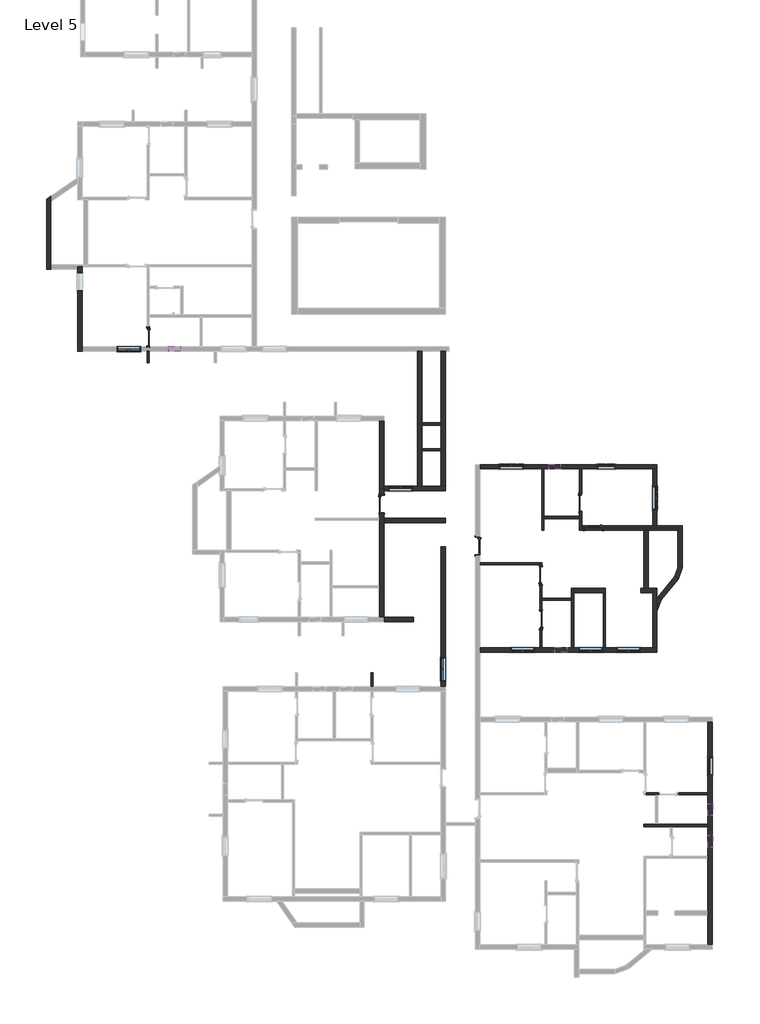
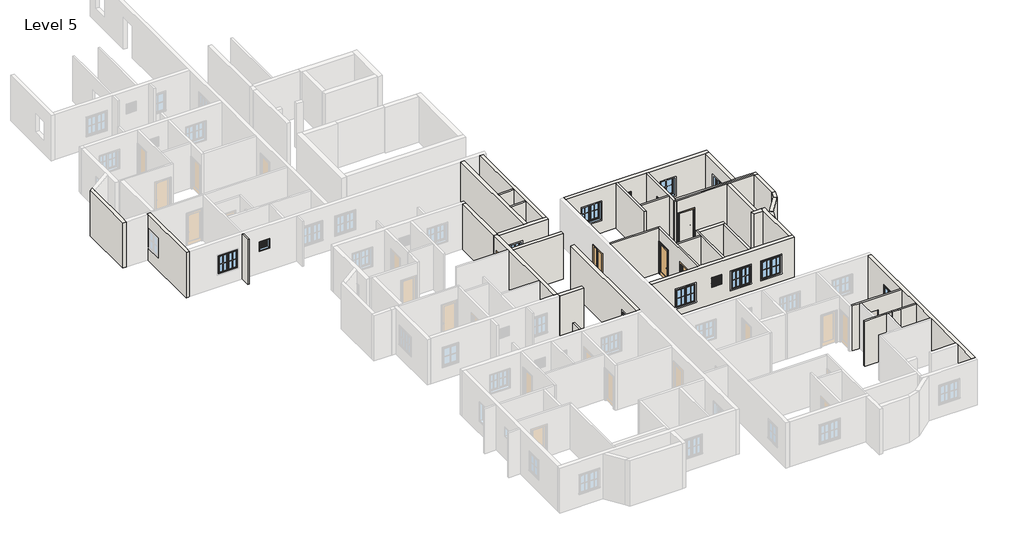
# One storey, part 3 of 7: 39 walls, 15 windows, 7 doors.
"""IFC4 building model written with IfcOpenShell, lengths in millimetres."""

from ifc_helpers import new_model, si_unit, point, frame, frame_2d, origin, place, context, project, spatial, polyline, circle_curve, trimmed, segment, composite_curve, outline, extrude, faceted_brep, transform, mapped, element, save
from components import door_3c6ab76a, door_a3feeac7, door_3b97b8e7, door_868ee8a9, window_272f20d6, window_casement_double_4_x_4_af3140d2, window_f2d8fef0

model = new_model("IFC4")

# Units and contexts
model_context = context("Model", 3, world=origin())
ifc_project = project(units=[si_unit("LENGTHUNIT", "METRE", prefix="MILLI")], contexts=[model_context])

# Site, building, storey
site = spatial("IfcSite", under=ifc_project)
building = spatial("IfcBuilding", under=site)
storey = spatial("IfcBuildingStorey", under=building, Name="Level 5", Elevation=6400.8)

# Doors
placement = place(None, origin())
door_shape = door_3c6ab76a(model_context)
element("IfcDoor", 1, ObjectType="Door-Interior-Single-1_Panel-Wood : 2'6\" x 7' door", at=placement, inside=storey, context=model_context, shape_type="MappedRepresentation", body=[
    mapped(door_shape, transform((-11252.4759469, 2064.0461172, 6400.8), x_axis=(0.0, -1.0, 0.0), y_axis=(1.0, 0.0, 0.0), z_axis=(0.0, 0.0, 1.0))),
])
door_2_shape = door_a3feeac7(model_context)
element("IfcDoor", 2, ObjectType="Door-Interior-Single-1_Panel-Wood : 2'6\" x 7' door", at=placement, inside=storey, context=model_context, shape_type="MappedRepresentation", body=[
    mapped(door_2_shape, transform((11042.3740531, -6465.2997229, 6400.8), x_axis=(0.0, -1.0, 0.0), y_axis=(1.0, 0.0, 0.0), z_axis=(0.0, 0.0, 1.0))),
])
element("IfcDoor", 3, ObjectType="Door-Interior-Single-1_Panel-Wood : 2'6\" x 7' door", at=placement, inside=storey, context=model_context, shape_type="MappedRepresentation", body=[
    mapped(door_2_shape, transform((9004.0240531, -12510.4997229, 6400.8), x_axis=(0.0, 1.0, 0.0), y_axis=(-1.0, 0.0, 0.0), z_axis=(0.0, 0.0, 1.0))),
])
element("IfcDoor", 4, ObjectType="Door-Interior-Single-1_Panel-Wood : 36\" x 84\"", at=placement, inside=storey, context=model_context, shape_type="MappedRepresentation", body=[
    mapped(door_shape, transform((8997.6740531, -10224.4997229, 6400.8), x_axis=(0.0, 1.0, 0.0), y_axis=(-1.0, 0.0, 0.0), z_axis=(0.0, 0.0, 1.0))),
])
door_3_shape = door_3b97b8e7(model_context)
element("IfcDoor", 5, ObjectType="Door-Interior-Single-1_Panel-Wood : 36\" x 84\"", at=placement, inside=storey, context=model_context, shape_type="MappedRepresentation", body=[
    mapped(door_3_shape, transform((5733.7740531, -8700.4997229, 6400.8), x_axis=(0.0, -1.0, 0.0), y_axis=(1.0, 0.0, 0.0), z_axis=(0.0, 0.0, 1.0))),
])
door_4_shape = door_868ee8a9(model_context)
element("IfcDoor", 6, ObjectType="Door-Interior-Single-1_Panel-Wood : 36\" x 84\"", at=placement, inside=storey, context=model_context, shape_type="MappedRepresentation", body=[
    mapped(door_4_shape, transform((787.1240531, -6537.0288828, 6400.8), x_axis=(0.0, -1.0, 0.0), y_axis=(1.0, 0.0, 0.0), z_axis=(0.0, 0.0, 1.0))),
])
element("IfcDoor", 7, ObjectType="Door-Interior-Single-1_Panel-Wood : 36\" x 84\"", at=placement, inside=storey, context=model_context, shape_type="MappedRepresentation", body=[
    mapped(door_4_shape, transform((11712.2990531, -7776.5747229, 6400.8), x_axis=(-1.0, 0.0, 0.0), y_axis=(0.0, -1.0, 0.0), z_axis=(0.0, 0.0, 1.0))),
])

# Walls
element("IfcWall", 8, ObjectType="4.5\" wall", at=placement, inside=storey, context=model_context, shape_type="SweptSolid", body=[
    extrude(outline(polyline([(-11312.8009469, 730.5461172), (-11312.8009469, 1340.1461172), (-11198.5009469, 1340.1461172), (-11198.5009469, 730.5461172), (-11312.8009469, 730.5461172)])), frame((0.0, 0.0, 6400.8), z_axis=(0.0, 0.0, 1.0), x_axis=(1.0, 0.0, 0.0)), (0.0, 0.0, 1.0), 3048.0),
])
element("IfcWall", 9, ObjectType="4.5\" wall", at=placement, inside=storey, context=model_context, shape_type="SweptSolid", body=[
    extrude(outline(polyline([(3850.9990531, -3803.3538828), (2860.3990531, -3803.3538828), (2860.3990531, -3689.0538828), (3850.9990531, -3689.0538828), (3850.9990531, -3803.3538828)])), frame((0.0, 0.0, 6400.8), z_axis=(0.0, 0.0, 1.0), x_axis=(1.0, 0.0, 0.0)), (0.0, 0.0, 1.0), 3048.0),
])
element("IfcWall", 10, ObjectType="4.5\" wall", at=placement, inside=storey, context=model_context, shape_type="SweptSolid", body=[
    extrude(outline(polyline([(2860.3990531, -2355.5538828), (3850.9990531, -2355.5538828), (3850.9990531, -2469.8538828), (2860.3990531, -2469.8538828), (2860.3990531, -2355.5538828)])), frame((0.0, 0.0, 6400.8), z_axis=(0.0, 0.0, 1.0), x_axis=(1.0, 0.0, 0.0)), (0.0, 0.0, 1.0), 3048.0),
])
element("IfcWall", 11, ObjectType="4.5\" wall", at=placement, inside=storey, context=model_context, shape_type="SweptSolid", body=[
    extrude(outline(polyline([(345.7990531, -15233.3538828), (345.7990531, -15957.2538828), (231.4990531, -15957.2538828), (231.4990531, -15233.3538828), (345.7990531, -15233.3538828)])), frame((0.0, 0.0, 6400.8), z_axis=(0.0, 0.0, 1.0), x_axis=(1.0, 0.0, 0.0)), (0.0, 0.0, 1.0), 3048.0),
])
element("IfcWall", 12, ObjectType="4.5\" wall", at=placement, inside=storey, context=model_context, shape_type="Brep", body=[
    faceted_brep([(17617.7990531, -21521.1497229, 9448.8), (15026.9990531, -21521.1497229, 9448.8), (14912.6990531, -21521.1497229, 9448.8), (14417.3990531, -21521.1497229, 9448.8), (14417.3990531, -21521.1497229, 6400.8), (14912.6990531, -21521.1497229, 6400.8), (15026.9990531, -21521.1497229, 6400.8), (15096.8490531, -21521.1497229, 6400.8), (15096.8490531, -21521.1497229, 8559.8), (16062.0490531, -21521.1497229, 8559.8), (16062.0490531, -21521.1497229, 6400.8), (17617.7990531, -21521.1497229, 6400.8), (14417.3990531, -21406.8497229, 9448.8), (17617.7990531, -21406.8497229, 9448.8), (17617.7990531, -21406.8497229, 6400.8), (16062.0490531, -21406.8497229, 6400.8), (16062.0490531, -21406.8497229, 8559.8), (15096.8490531, -21406.8497229, 8559.8), (15096.8490531, -21406.8497229, 6400.8), (14417.3990531, -21406.8497229, 6400.8)], [[[0, 1, 2, 3, 4, 5, 6, 7, 8, 9, 10, 11]], [[12, 13, 14, 15, 16, 17, 18, 19]], [[14, 11, 10, 15]], [[4, 19, 18, 7, 6, 5]], [[3, 2, 1, 0, 13, 12]], [[0, 11, 14, 13]], [[4, 3, 12, 19]], [[17, 8, 7, 18]], [[8, 17, 16, 9]], [[9, 16, 15, 10]]]),
])
element("IfcWall", 13, ObjectType="4.5\" wall", at=placement, inside=storey, context=model_context, shape_type="SweptSolid", body=[
    extrude(outline(polyline([(16055.6990531, -23045.1497229), (16589.0990531, -23045.1497229), (16589.0990531, -23159.4497229), (16055.6990531, -23159.4497229), (16055.6990531, -23045.1497229)])), frame((0.0, 0.0, 6400.8), z_axis=(0.0, 0.0, 1.0), x_axis=(1.0, 0.0, 0.0)), (0.0, 0.0, 1.0), 3048.0),
])
element("IfcWall", 14, ObjectType="4.5\" wall", at=placement, inside=storey, context=model_context, shape_type="Brep", body=[
    faceted_brep([(17617.7990531, -23045.1497229, 6400.8), (15026.9990531, -23045.1497229, 6400.8), (14912.6990531, -23045.1497229, 6400.8), (14303.0990531, -23045.1497229, 6400.8), (14303.0990531, -23045.1497229, 9448.8), (14912.6990531, -23045.1497229, 9448.8), (15026.9990531, -23045.1497229, 9448.8), (17617.7990531, -23045.1497229, 9448.8), (17617.7990531, -23159.4497229, 6400.8), (17617.7990531, -23159.4497229, 9448.8), (15788.9990531, -23159.4497229, 9448.8), (15674.6990531, -23159.4497229, 9448.8), (14303.0990531, -23159.4497229, 9448.8), (14303.0990531, -23159.4497229, 6400.8), (15674.6990531, -23159.4497229, 6400.8), (15788.9990531, -23159.4497229, 6400.8)], [[[0, 1, 2, 3, 4, 5, 6, 7]], [[8, 9, 10, 11, 12, 13, 14, 15]], [[3, 2, 1, 0, 8, 15, 14, 13]], [[4, 3, 13, 12]], [[7, 6, 5, 4, 12, 11, 10, 9]], [[0, 7, 9, 8]]]),
])
element("IfcWall", 15, ObjectType="4.5\" wall", at=placement, inside=storey, context=model_context, shape_type="Brep", body=[
    faceted_brep([(10988.3990531, -7894.0497229, 6400.8), (14303.0990531, -7894.0497229, 6400.8), (14531.6990531, -7894.0497229, 6400.8), (16055.6990531, -7894.0497229, 6400.8), (16055.6990531, -7894.0497229, 9448.8), (14531.6990531, -7894.0497229, 9448.8), (14303.0990531, -7894.0497229, 9448.8), (10988.3990531, -7894.0497229, 9448.8), (10988.3990531, -7779.7497229, 6400.8), (10988.3990531, -7779.7497229, 9448.8), (11102.6990531, -7779.7497229, 9448.8), (16055.6990531, -7779.7497229, 9448.8), (16055.6990531, -7779.7497229, 6400.8), (11102.6990531, -7779.7497229, 6400.8)], [[[0, 1, 2, 3, 4, 5, 6, 7]], [[8, 9, 10, 11, 12, 13]], [[3, 2, 1, 0, 8, 13, 12]], [[7, 6, 5, 4, 11, 10, 9]], [[0, 7, 9, 8]], [[4, 3, 12, 11]]]),
])
element("IfcWall", 16, ObjectType="4.5\" wall", at=placement, inside=storey, context=model_context, shape_type="Brep", body=[
    faceted_brep([(10696.2990531, -13939.2497229, 6400.8), (10696.2990531, -11119.8497229, 6400.8), (10696.2990531, -10891.2497229, 6400.8), (10696.2990531, -10891.2497229, 9448.8), (10696.2990531, -11119.8497229, 9448.8), (10696.2990531, -13939.2497229, 9448.8), (10581.9990531, -13939.2497229, 6400.8), (10581.9990531, -13939.2497229, 9448.8), (10581.9990531, -11500.8497229, 9448.8), (10581.9990531, -11386.5497229, 9448.8), (10581.9990531, -10891.2497229, 9448.8), (10581.9990531, -10891.2497229, 6400.8), (10581.9990531, -11386.5497229, 6400.8), (10581.9990531, -11500.8497229, 6400.8)], [[[0, 1, 2, 3, 4, 5]], [[6, 7, 8, 9, 10, 11, 12, 13]], [[2, 1, 0, 6, 13, 12, 11]], [[5, 4, 3, 10, 9, 8, 7]], [[0, 5, 7, 6]], [[3, 2, 11, 10]]]),
])
element("IfcWall", 17, ObjectType="4.5\" wall", at=placement, inside=storey, context=model_context, shape_type="SweptSolid", body=[
    extrude(outline(polyline([(9057.9990531, -11386.5497229), (10581.9990531, -11386.5497229), (10581.9990531, -11500.8497229), (9057.9990531, -11500.8497229), (9057.9990531, -11386.5497229)])), frame((0.0, 0.0, 6400.8), z_axis=(0.0, 0.0, 1.0), x_axis=(1.0, 0.0, 0.0)), (0.0, 0.0, 1.0), 3048.0),
])
element("IfcWall", 18, ObjectType="4.5\" wall", at=placement, inside=storey, context=model_context, shape_type="Brep", body=[
    faceted_brep([(8943.6990531, -13939.2497229, 9448.8), (8943.6990531, -9672.0497229, 9448.8), (8943.6990531, -9557.7497229, 9448.8), (8943.6990531, -9557.7497229, 6400.8), (8943.6990531, -9672.0497229, 6400.8), (8943.6990531, -9741.8997229, 6400.8), (8943.6990531, -9741.8997229, 8559.8), (8943.6990531, -10707.0997229, 8559.8), (8943.6990531, -10707.0997229, 6400.8), (8943.6990531, -12027.8997229, 6400.8), (8943.6990531, -12027.8997229, 8559.8), (8943.6990531, -12993.0997229, 8559.8), (8943.6990531, -12993.0997229, 6400.8), (8943.6990531, -13939.2497229, 6400.8), (9057.9990531, -9557.7497229, 9448.8), (9057.9990531, -11386.5497229, 9448.8), (9057.9990531, -11500.8497229, 9448.8), (9057.9990531, -13939.2497229, 9448.8), (9057.9990531, -13939.2497229, 6400.8), (9057.9990531, -12993.0997229, 6400.8), (9057.9990531, -12993.0997229, 8559.8), (9057.9990531, -12027.8997229, 8559.8), (9057.9990531, -12027.8997229, 6400.8), (9057.9990531, -11500.8497229, 6400.8), (9057.9990531, -11386.5497229, 6400.8), (9057.9990531, -10707.0997229, 6400.8), (9057.9990531, -10707.0997229, 8559.8), (9057.9990531, -9741.8997229, 8559.8), (9057.9990531, -9741.8997229, 6400.8), (9057.9990531, -9557.7497229, 6400.8)], [[[0, 1, 2, 3, 4, 5, 6, 7, 8, 9, 10, 11, 12, 13]], [[14, 15, 16, 17, 18, 19, 20, 21, 22, 23, 24, 25, 26, 27, 28, 29]], [[18, 13, 12, 19]], [[3, 29, 28, 5, 4]], [[22, 9, 8, 25, 24, 23]], [[2, 1, 0, 17, 16, 15, 14]], [[0, 13, 18, 17]], [[3, 2, 14, 29]], [[21, 10, 9, 22]], [[10, 21, 20, 11]], [[11, 20, 19, 12]], [[27, 6, 5, 28]], [[6, 27, 26, 7]], [[7, 26, 25, 8]]]),
])
element("IfcWall", 19, ObjectType="4.5\" wall", at=placement, inside=storey, context=model_context, shape_type="SweptSolid", body=[
    extrude(outline(polyline([(8943.6990531, -9672.0497229), (5844.8990531, -9672.0497229), (5844.8990531, -9557.7497229), (8943.6990531, -9557.7497229), (8943.6990531, -9672.0497229)])), frame((0.0, 0.0, 6400.8), z_axis=(0.0, 0.0, 1.0), x_axis=(1.0, 0.0, 0.0)), (0.0, 0.0, 1.0), 3048.0),
])
element("IfcWall", 20, ObjectType="4.5\" wall", at=placement, inside=storey, context=model_context, shape_type="Brep", body=[
    faceted_brep([(9045.2990531, -4731.7497229, 6400.8), (9045.2990531, -7894.0497229, 6400.8), (9045.2990531, -7894.0497229, 9448.8), (9045.2990531, -4731.7497229, 9448.8), (9159.5990531, -4731.7497229, 6400.8), (9159.5990531, -4731.7497229, 9448.8), (9159.5990531, -7170.1497229, 9448.8), (9159.5990531, -7284.4497229, 9448.8), (9159.5990531, -7894.0497229, 9448.8), (9159.5990531, -7894.0497229, 6400.8), (9159.5990531, -7284.4497229, 6400.8), (9159.5990531, -7170.1497229, 6400.8)], [[[0, 1, 2, 3]], [[4, 5, 6, 7, 8, 9, 10, 11]], [[1, 0, 4, 11, 10, 9]], [[2, 1, 9, 8]], [[3, 2, 8, 7, 6, 5]], [[0, 3, 5, 4]]]),
])
element("IfcWall", 21, ObjectType="4.5\" wall", at=placement, inside=storey, context=model_context, shape_type="Brep", body=[
    faceted_brep([(10988.3990531, -7779.7497229, 9448.8), (10988.3990531, -7284.4497229, 9448.8), (10988.3990531, -7170.1497229, 9448.8), (10988.3990531, -4731.7497229, 9448.8), (10988.3990531, -4731.7497229, 6400.8), (10988.3990531, -5982.6997229, 6400.8), (10988.3990531, -5982.6997229, 8559.8), (10988.3990531, -6947.8997229, 8559.8), (10988.3990531, -6947.8997229, 6400.8), (10988.3990531, -7170.1497229, 6400.8), (10988.3990531, -7284.4497229, 6400.8), (10988.3990531, -7779.7497229, 6400.8), (11102.6990531, -4731.7497229, 9448.8), (11102.6990531, -7665.4497229, 9448.8), (11102.6990531, -7779.7497229, 9448.8), (11102.6990531, -7779.7497229, 6400.8), (11102.6990531, -7665.4497229, 6400.8), (11102.6990531, -6947.8997229, 6400.8), (11102.6990531, -6947.8997229, 8559.8), (11102.6990531, -5982.6997229, 8559.8), (11102.6990531, -5982.6997229, 6400.8), (11102.6990531, -4731.7497229, 6400.8)], [[[0, 1, 2, 3, 4, 5, 6, 7, 8, 9, 10, 11]], [[12, 13, 14, 15, 16, 17, 18, 19, 20, 21]], [[4, 21, 20, 5]], [[15, 11, 10, 9, 8, 17, 16]], [[3, 2, 1, 0, 14, 13, 12]], [[4, 3, 12, 21]], [[0, 11, 15, 14]], [[7, 18, 17, 8]], [[18, 7, 6, 19]], [[19, 6, 5, 20]]]),
])
element("IfcWall", 22, ObjectType="4.5\" wall", at=placement, inside=storey, context=model_context, shape_type="SweptSolid", body=[
    extrude(outline(polyline([(10988.3990531, -7284.4497229), (9159.5990531, -7284.4497229), (9159.5990531, -7170.1497229), (10988.3990531, -7170.1497229), (10988.3990531, -7284.4497229)])), frame((0.0, 0.0, 6400.8), z_axis=(0.0, 0.0, 1.0), x_axis=(1.0, 0.0, 0.0)), (0.0, 0.0, 1.0), 3048.0),
])
element("IfcWall", 23, ObjectType="4.5\" wall", at=placement, inside=storey, context=model_context, shape_type="SweptSolid", body=[
    extrude(outline(polyline([(12220.2990531, -13939.2497229), (12220.2990531, -11119.8497229), (12334.5990531, -11119.8497229), (12334.5990531, -13939.2497229), (12220.2990531, -13939.2497229)])), frame((0.0, 0.0, 6400.8), z_axis=(0.0, 0.0, 1.0), x_axis=(1.0, 0.0, 0.0)), (0.0, 0.0, 1.0), 3048.0),
])
element("IfcWall", 24, ObjectType="9\"", at=placement, inside=storey, context=model_context, shape_type="Brep", body=[
    faceted_brep([(-14894.2009469, 5683.5461172, 6400.8), (-14894.2009469, 5569.2461172, 6400.8), (-14894.2009469, 1340.1461172, 6400.8), (-14894.2009469, 1340.1461172, 9448.8), (-14894.2009469, 5569.2461172, 9448.8), (-14894.2009469, 5683.5461172, 9448.8), (-14894.2009469, 5378.7461172, 8534.4), (-14894.2009469, 4464.3461172, 8534.4), (-14894.2009469, 4464.3461172, 7315.2), (-14894.2009469, 5378.7461172, 7315.2), (-14665.6009469, 5683.5461172, 6400.8), (-14665.6009469, 5683.5461172, 9448.8), (-14665.6009469, 1568.7461172, 9448.8), (-14665.6009469, 1340.1461172, 9448.8), (-14665.6009469, 1340.1461172, 6400.8), (-14665.6009469, 1568.7461172, 6400.8), (-14665.6009469, 5378.7461172, 8534.4), (-14665.6009469, 5378.7461172, 7315.2), (-14665.6009469, 4464.3461172, 7315.2), (-14665.6009469, 4464.3461172, 8534.4)], [[[0, 1, 2, 3, 4, 5], [6, 7, 8, 9]], [[10, 11, 12, 13, 14, 15], [16, 17, 18, 19]], [[2, 1, 0, 10, 15, 14]], [[5, 4, 3, 13, 12, 11]], [[3, 2, 14, 13]], [[0, 5, 11, 10]], [[17, 16, 6, 9]], [[18, 17, 9, 8]], [[19, 18, 8, 7]], [[16, 19, 7, 6]]]),
])
element("IfcWall", 25, ObjectType="9\"", at=placement, inside=storey, context=model_context, shape_type="Brep", body=[
    faceted_brep([(904.5990531, -5746.4538828, 6400.8), (904.5990531, -5632.1538828, 6400.8), (904.5990531, -2241.2538828, 6400.8), (904.5990531, -2241.2538828, 9448.8), (904.5990531, -5632.1538828, 9448.8), (904.5990531, -5746.4538828, 9448.8), (675.9990531, -5746.4538828, 6400.8), (675.9990531, -5746.4538828, 9448.8), (675.9990531, -2241.2538828, 9448.8), (675.9990531, -2241.2538828, 6400.8)], [[[0, 1, 2, 3, 4, 5]], [[6, 7, 8, 9]], [[2, 1, 0, 6, 9]], [[5, 4, 3, 8, 7]], [[0, 5, 7, 6]], [[3, 2, 9, 8]]]),
])
element("IfcWall", 26, ObjectType="9\"", at=placement, inside=storey, context=model_context, shape_type="Brep", body=[
    faceted_brep([(904.5990531, -5746.4538828, 6400.8), (904.5990531, -5746.4538828, 9448.8), (904.5990531, -5860.7538828, 9448.8), (904.5990531, -7270.4538828, 9448.8), (904.5990531, -7499.0538828, 9448.8), (904.5990531, -12375.8538828, 9448.8), (904.5990531, -12375.8538828, 6400.8), (904.5990531, -7499.0538828, 6400.8), (904.5990531, -7270.4538828, 6400.8), (904.5990531, -7019.6288828, 6400.8), (904.5990531, -7019.6288828, 8559.8), (904.5990531, -6054.4288828, 8559.8), (904.5990531, -6054.4288828, 6400.8), (904.5990531, -5860.7538828, 6400.8), (675.9990531, -5746.4538828, 9448.8), (675.9990531, -5746.4538828, 6400.8), (675.9990531, -6054.4288828, 6400.8), (675.9990531, -6054.4288828, 8559.8), (675.9990531, -7019.6288828, 8559.8), (675.9990531, -7019.6288828, 6400.8), (675.9990531, -7270.4538828, 6400.8), (675.9990531, -7384.7538828, 6400.8), (675.9990531, -10737.5538828, 6400.8), (675.9990531, -10851.8538828, 6400.8), (675.9990531, -12375.8538828, 6400.8), (675.9990531, -12375.8538828, 9448.8), (675.9990531, -10851.8538828, 9448.8), (675.9990531, -10737.5538828, 9448.8), (675.9990531, -7384.7538828, 9448.8), (675.9990531, -7270.4538828, 9448.8)], [[[0, 1, 2, 3, 4, 5, 6, 7, 8, 9, 10, 11, 12, 13]], [[14, 15, 16, 17, 18, 19, 20, 21, 22, 23, 24, 25, 26, 27, 28, 29]], [[6, 24, 23, 22, 21, 20, 19, 9, 8, 7]], [[15, 0, 13, 12, 16]], [[1, 0, 15, 14]], [[5, 4, 3, 2, 1, 14, 29, 28, 27, 26, 25]], [[6, 5, 25, 24]], [[18, 10, 9, 19]], [[10, 18, 17, 11]], [[11, 17, 16, 12]]]),
])
element("IfcWall", 27, ObjectType="9\"", at=placement, inside=storey, context=model_context, shape_type="SweptSolid", body=[
    extrude(outline(polyline([(904.5990531, -7270.4538828), (4079.5990531, -7270.4538828), (4079.5990531, -7499.0538828), (904.5990531, -7499.0538828), (904.5990531, -7270.4538828)])), frame((0.0, 0.0, 6400.8), z_axis=(0.0, 0.0, 1.0), x_axis=(1.0, 0.0, 0.0)), (0.0, 0.0, 1.0), 3048.0),
])
element("IfcWall", 28, ObjectType="9\"", at=placement, inside=storey, context=model_context, shape_type="Brep", body=[
    faceted_brep([(904.5990531, -5860.7538828, 6400.8), (4079.5990531, -5860.7538828, 6400.8), (4079.5990531, -5860.7538828, 9448.8), (904.5990531, -5860.7538828, 9448.8), (2377.7990531, -5860.7538828, 8534.4), (2377.7990531, -5860.7538828, 7315.2), (1158.5990531, -5860.7538828, 7315.2), (1158.5990531, -5860.7538828, 8534.4), (904.5990531, -5632.1538828, 6400.8), (904.5990531, -5632.1538828, 9448.8), (2631.7990531, -5632.1538828, 9448.8), (2860.3990531, -5632.1538828, 9448.8), (3850.9990531, -5632.1538828, 9448.8), (4079.5990531, -5632.1538828, 9448.8), (4079.5990531, -5632.1538828, 6400.8), (3850.9990531, -5632.1538828, 6400.8), (2860.3990531, -5632.1538828, 6400.8), (2631.7990531, -5632.1538828, 6400.8), (2377.7990531, -5632.1538828, 8534.4), (1158.5990531, -5632.1538828, 8534.4), (1158.5990531, -5632.1538828, 7315.2), (2377.7990531, -5632.1538828, 7315.2), (904.5990531, -5746.4538828, 6400.8), (904.5990531, -5746.4538828, 9448.8)], [[[0, 1, 2, 3], [4, 5, 6, 7]], [[8, 9, 10, 11, 12, 13, 14, 15, 16, 17], [18, 19, 20, 21]], [[1, 0, 22, 8, 17, 16, 15, 14]], [[3, 2, 13, 12, 11, 10, 9, 23]], [[0, 3, 23, 9, 8, 22]], [[2, 1, 14, 13]], [[5, 4, 18, 21]], [[6, 5, 21, 20]], [[7, 6, 20, 19]], [[4, 7, 19, 18]]]),
])
element("IfcWall", 29, ObjectType="9\"", at=placement, inside=storey, context=model_context, shape_type="Brep", body=[
    faceted_brep([(2631.7990531, 1340.1461172, 6400.8), (2631.7990531, -5632.1538828, 6400.8), (2631.7990531, -5632.1538828, 9448.8), (2631.7990531, 1340.1461172, 9448.8), (2860.3990531, 1340.1461172, 6400.8), (2860.3990531, 1340.1461172, 9448.8), (2860.3990531, -2355.5538828, 9448.8), (2860.3990531, -2469.8538828, 9448.8), (2860.3990531, -3689.0538828, 9448.8), (2860.3990531, -3803.3538828, 9448.8), (2860.3990531, -5632.1538828, 9448.8), (2860.3990531, -5632.1538828, 6400.8), (2860.3990531, -3803.3538828, 6400.8), (2860.3990531, -3689.0538828, 6400.8), (2860.3990531, -2469.8538828, 6400.8), (2860.3990531, -2355.5538828, 6400.8)], [[[0, 1, 2, 3]], [[4, 5, 6, 7, 8, 9, 10, 11, 12, 13, 14, 15]], [[1, 0, 4, 15, 14, 13, 12, 11]], [[3, 2, 10, 9, 8, 7, 6, 5]], [[0, 3, 5, 4]], [[2, 1, 11, 10]]]),
])
element("IfcWall", 30, ObjectType="9\"", at=placement, inside=storey, context=model_context, shape_type="Brep", body=[
    faceted_brep([(4079.5990531, -5632.1538828, 6400.8), (4079.5990531, 1340.1461172, 6400.8), (4079.5990531, 1340.1461172, 9448.8), (4079.5990531, -5632.1538828, 9448.8), (3850.9990531, -5632.1538828, 6400.8), (3850.9990531, -5632.1538828, 9448.8), (3850.9990531, -3803.3538828, 9448.8), (3850.9990531, -3689.0538828, 9448.8), (3850.9990531, -2469.8538828, 9448.8), (3850.9990531, -2355.5538828, 9448.8), (3850.9990531, 1340.1461172, 9448.8), (3850.9990531, 1340.1461172, 6400.8), (3850.9990531, -2355.5538828, 6400.8), (3850.9990531, -2469.8538828, 6400.8), (3850.9990531, -3689.0538828, 6400.8), (3850.9990531, -3803.3538828, 6400.8)], [[[0, 1, 2, 3]], [[4, 5, 6, 7, 8, 9, 10, 11, 12, 13, 14, 15]], [[1, 0, 4, 15, 14, 13, 12, 11]], [[3, 2, 10, 9, 8, 7, 6, 5]], [[2, 1, 11, 10]], [[0, 3, 5, 4]]]),
])
element("IfcWall", 31, ObjectType="9\"", at=placement, inside=storey, context=model_context, shape_type="SweptSolid", body=[
    extrude(outline(polyline([(904.5990531, -12375.8538828), (2441.2990531, -12375.8538828), (2441.2990531, -12604.4538828), (904.5990531, -12604.4538828), (904.5990531, -12375.8538828)])), frame((0.0, 0.0, 6400.8), z_axis=(0.0, 0.0, 1.0), x_axis=(1.0, 0.0, 0.0)), (0.0, 0.0, 1.0), 3048.0),
])
element("IfcWall", 32, ObjectType="9\"", at=placement, inside=storey, context=model_context, shape_type="Brep", body=[
    faceted_brep([(17617.7990531, -17749.2497229, 6400.8), (17617.7990531, -21406.8497229, 6400.8), (17617.7990531, -21521.1497229, 6400.8), (17617.7990531, -23045.1497229, 6400.8), (17617.7990531, -23159.4497229, 6400.8), (17617.7990531, -24683.4497229, 6400.8), (17617.7990531, -24797.7497229, 6400.8), (17617.7990531, -27502.8497229, 6400.8), (17617.7990531, -27731.4497229, 6400.8), (17617.7990531, -29255.4497229, 6400.8), (17617.7990531, -29255.4497229, 9448.8), (17617.7990531, -27731.4497229, 9448.8), (17617.7990531, -27502.8497229, 9448.8), (17617.7990531, -24797.7497229, 9448.8), (17617.7990531, -24683.4497229, 9448.8), (17617.7990531, -23159.4497229, 9448.8), (17617.7990531, -23045.1497229, 9448.8), (17617.7990531, -21521.1497229, 9448.8), (17617.7990531, -21406.8497229, 9448.8), (17617.7990531, -17749.2497229, 9448.8), (17617.7990531, -22587.9497229, 8534.4), (17617.7990531, -22587.9497229, 7924.8), (17617.7990531, -21978.3497229, 7924.8), (17617.7990531, -21978.3497229, 8534.4), (17617.7990531, -23616.6497229, 8534.4), (17617.7990531, -24226.2497229, 8534.4), (17617.7990531, -24226.2497229, 7924.8), (17617.7990531, -23616.6497229, 7924.8), (17617.7990531, -19584.3997229, 8534.4), (17617.7990531, -20498.7997229, 8534.4), (17617.7990531, -20498.7997229, 7315.2), (17617.7990531, -19584.3997229, 7315.2), (17846.3990531, -17749.2497229, 6400.8), (17846.3990531, -17749.2497229, 9448.8), (17846.3990531, -29255.4497229, 9448.8), (17846.3990531, -29255.4497229, 6400.8), (17846.3990531, -22587.9497229, 8534.4), (17846.3990531, -21978.3497229, 8534.4), (17846.3990531, -21978.3497229, 7924.8), (17846.3990531, -22587.9497229, 7924.8), (17846.3990531, -23616.6497229, 8534.4), (17846.3990531, -23616.6497229, 7924.8), (17846.3990531, -24226.2497229, 7924.8), (17846.3990531, -24226.2497229, 8534.4), (17846.3990531, -19584.3997229, 8534.4), (17846.3990531, -19584.3997229, 7315.2), (17846.3990531, -20498.7997229, 7315.2), (17846.3990531, -20498.7997229, 8534.4)], [[[0, 1, 2, 3, 4, 5, 6, 7, 8, 9, 10, 11, 12, 13, 14, 15, 16, 17, 18, 19], [20, 21, 22, 23], [24, 25, 26, 27], [28, 29, 30, 31]], [[32, 33, 34, 35], [36, 37, 38, 39], [40, 41, 42, 43], [44, 45, 46, 47]], [[9, 8, 7, 6, 5, 4, 3, 2, 1, 0, 32, 35]], [[19, 18, 17, 16, 15, 14, 13, 12, 11, 10, 34, 33]], [[0, 19, 33, 32]], [[10, 9, 35, 34]], [[21, 20, 36, 39]], [[22, 21, 39, 38]], [[23, 22, 38, 37]], [[20, 23, 37, 36]], [[41, 40, 24, 27]], [[42, 41, 27, 26]], [[43, 42, 26, 25]], [[40, 43, 25, 24]], [[45, 44, 28, 31]], [[46, 45, 31, 30]], [[47, 46, 30, 29]], [[44, 47, 29, 28]]]),
])
element("IfcWall", 33, ObjectType="9\"", at=placement, inside=storey, context=model_context, shape_type="Brep", body=[
    faceted_brep([(5844.8990531, -14167.8497229, 6400.8), (14988.8990531, -14167.8497229, 6400.8), (14988.8990531, -14167.8497229, 9448.8), (5844.8990531, -14167.8497229, 9448.8), (10334.3490531, -14167.8497229, 8534.4), (10334.3490531, -14167.8497229, 7924.8), (9724.7490531, -14167.8497229, 7924.8), (9724.7490531, -14167.8497229, 8534.4), (12912.4490531, -14167.8497229, 8534.4), (14131.6490531, -14167.8497229, 8534.4), (14131.6490531, -14167.8497229, 7315.2), (12912.4490531, -14167.8497229, 7315.2), (10956.6490531, -14167.8497229, 8534.4), (12175.8490531, -14167.8497229, 8534.4), (12175.8490531, -14167.8497229, 7315.2), (10956.6490531, -14167.8497229, 7315.2), (7451.4490531, -14167.8497229, 8534.4), (8670.6490531, -14167.8497229, 8534.4), (8670.6490531, -14167.8497229, 7315.2), (7451.4490531, -14167.8497229, 7315.2), (5844.8990531, -13939.2497229, 6400.8), (5844.8990531, -13939.2497229, 9448.8), (8943.6990531, -13939.2497229, 9448.8), (9057.9990531, -13939.2497229, 9448.8), (10581.9990531, -13939.2497229, 9448.8), (10696.2990531, -13939.2497229, 9448.8), (12220.2990531, -13939.2497229, 9448.8), (12334.5990531, -13939.2497229, 9448.8), (14760.2990531, -13939.2497229, 9448.8), (14988.8990531, -13939.2497229, 9448.8), (14988.8990531, -13939.2497229, 6400.8), (14760.2990531, -13939.2497229, 6400.8), (12334.5990531, -13939.2497229, 6400.8), (12220.2990531, -13939.2497229, 6400.8), (10696.2990531, -13939.2497229, 6400.8), (10581.9990531, -13939.2497229, 6400.8), (9057.9990531, -13939.2497229, 6400.8), (8943.6990531, -13939.2497229, 6400.8), (10334.3490531, -13939.2497229, 8534.4), (9724.7490531, -13939.2497229, 8534.4), (9724.7490531, -13939.2497229, 7924.8), (10334.3490531, -13939.2497229, 7924.8), (12912.4490531, -13939.2497229, 8534.4), (12912.4490531, -13939.2497229, 7315.2), (14131.6490531, -13939.2497229, 7315.2), (14131.6490531, -13939.2497229, 8534.4), (10956.6490531, -13939.2497229, 8534.4), (10956.6490531, -13939.2497229, 7315.2), (12175.8490531, -13939.2497229, 7315.2), (12175.8490531, -13939.2497229, 8534.4), (7451.4490531, -13939.2497229, 8534.4), (7451.4490531, -13939.2497229, 7315.2), (8670.6490531, -13939.2497229, 7315.2), (8670.6490531, -13939.2497229, 8534.4)], [[[0, 1, 2, 3], [4, 5, 6, 7], [8, 9, 10, 11], [12, 13, 14, 15], [16, 17, 18, 19]], [[20, 21, 22, 23, 24, 25, 26, 27, 28, 29, 30, 31, 32, 33, 34, 35, 36, 37], [38, 39, 40, 41], [42, 43, 44, 45], [46, 47, 48, 49], [50, 51, 52, 53]], [[1, 0, 20, 37, 36, 35, 34, 33, 32, 31, 30]], [[3, 2, 29, 28, 27, 26, 25, 24, 23, 22, 21]], [[0, 3, 21, 20]], [[2, 1, 30, 29]], [[5, 4, 38, 41]], [[6, 5, 41, 40]], [[7, 6, 40, 39]], [[4, 7, 39, 38]], [[43, 42, 8, 11]], [[44, 43, 11, 10]], [[45, 44, 10, 9]], [[42, 45, 9, 8]], [[47, 46, 12, 15]], [[48, 47, 15, 14]], [[49, 48, 14, 13]], [[46, 49, 13, 12]], [[51, 50, 16, 19]], [[52, 51, 19, 18]], [[53, 52, 18, 17]], [[50, 53, 17, 16]]]),
])
element("IfcWall", 34, ObjectType="9\"", at=placement, inside=storey, context=model_context, shape_type="SweptSolid", body=[
    extrude(outline(polyline([(-15957.2538828, 6400.8), (-15957.2538828, 9448.8), (-8732.9659091, 9448.8), (-8732.9659091, 6400.8), (-15957.2538828, 6400.8)]), holes=[polyline([(-14445.9538828, 8534.4), (-15665.1538828, 8534.4), (-15665.1538828, 7315.2), (-14445.9538828, 7315.2), (-14445.9538828, 8534.4)])]), frame((3850.9990531, 0.0, 0.0), z_axis=(1.0, 0.0, 0.0), x_axis=(0.0, 1.0, 0.0)), (0.0, 0.0, 1.0), 228.6),
])
element("IfcWall", 35, ObjectType="9\"", at=placement, inside=storey, context=model_context, shape_type="Brep", body=[
    faceted_brep([(5844.8990531, -4731.7497229, 6400.8), (9045.2990531, -4731.7497229, 6400.8), (9159.5990531, -4731.7497229, 6400.8), (10988.3990531, -4731.7497229, 6400.8), (11102.6990531, -4731.7497229, 6400.8), (14760.2990531, -4731.7497229, 6400.8), (14988.8990531, -4731.7497229, 6400.8), (14988.8990531, -4731.7497229, 9448.8), (14760.2990531, -4731.7497229, 9448.8), (11102.6990531, -4731.7497229, 9448.8), (10988.3990531, -4731.7497229, 9448.8), (9159.5990531, -4731.7497229, 9448.8), (9045.2990531, -4731.7497229, 9448.8), (5844.8990531, -4731.7497229, 9448.8), (10016.8490531, -4731.7497229, 8534.4), (10016.8490531, -4731.7497229, 7924.8), (9407.2490531, -4731.7497229, 7924.8), (9407.2490531, -4731.7497229, 8534.4), (12823.5490531, -4731.7497229, 8534.4), (12823.5490531, -4731.7497229, 7315.2), (11909.1490531, -4731.7497229, 7315.2), (11909.1490531, -4731.7497229, 8534.4), (8086.4490531, -4731.7497229, 8534.4), (8086.4490531, -4731.7497229, 7315.2), (6867.2490531, -4731.7497229, 7315.2), (6867.2490531, -4731.7497229, 8534.4), (5844.8990531, -4503.1497229, 6400.8), (5844.8990531, -4503.1497229, 9448.8), (14988.8990531, -4503.1497229, 9448.8), (14988.8990531, -4503.1497229, 6400.8), (10016.8490531, -4503.1497229, 8534.4), (9407.2490531, -4503.1497229, 8534.4), (9407.2490531, -4503.1497229, 7924.8), (10016.8490531, -4503.1497229, 7924.8), (12823.5490531, -4503.1497229, 8534.4), (11909.1490531, -4503.1497229, 8534.4), (11909.1490531, -4503.1497229, 7315.2), (12823.5490531, -4503.1497229, 7315.2), (8086.4490531, -4503.1497229, 8534.4), (6867.2490531, -4503.1497229, 8534.4), (6867.2490531, -4503.1497229, 7315.2), (8086.4490531, -4503.1497229, 7315.2)], [[[0, 1, 2, 3, 4, 5, 6, 7, 8, 9, 10, 11, 12, 13], [14, 15, 16, 17], [18, 19, 20, 21], [22, 23, 24, 25]], [[26, 27, 28, 29], [30, 31, 32, 33], [34, 35, 36, 37], [38, 39, 40, 41]], [[6, 5, 4, 3, 2, 1, 0, 26, 29]], [[13, 12, 11, 10, 9, 8, 7, 28, 27]], [[7, 6, 29, 28]], [[0, 13, 27, 26]], [[15, 14, 30, 33]], [[16, 15, 33, 32]], [[17, 16, 32, 31]], [[14, 17, 31, 30]], [[19, 18, 34, 37]], [[20, 19, 37, 36]], [[21, 20, 36, 35]], [[18, 21, 35, 34]], [[23, 22, 38, 41]], [[24, 23, 41, 40]], [[25, 24, 40, 39]], [[22, 25, 39, 38]]]),
])
element("IfcWall", 36, ObjectType="9\"", at=placement, inside=storey, context=model_context, shape_type="SweptSolid", body=[
    extrude(outline(polyline([(-7665.4497229, 6400.8), (-7665.4497229, 9448.8), (-4731.7497229, 9448.8), (-4731.7497229, 6400.8), (-7665.4497229, 6400.8)]), holes=[polyline([(-6836.7747229, 8534.4), (-6836.7747229, 7315.2), (-5617.5747229, 7315.2), (-5617.5747229, 8534.4), (-6836.7747229, 8534.4)])]), frame((14760.2990531, 0.0, 0.0), z_axis=(1.0, 0.0, 0.0), x_axis=(0.0, 1.0, 0.0)), (0.0, 0.0, 1.0), 228.6),
])
element("IfcWall", 37, ObjectType="9\"", at=placement, inside=storey, context=model_context, shape_type="Brep", body=[
    faceted_brep([(14988.8990531, -13939.2497229, 6400.8), (14988.8990531, -12059.0648255, 6400.8), (14988.8990531, -11373.2648255, 6400.8), (14988.8990531, -10891.2497229, 6400.8), (14988.8990531, -10891.2497229, 9448.8), (14988.8990531, -11373.2648255, 9448.8), (14988.8990531, -12059.0648255, 9448.8), (14988.8990531, -13939.2497229, 9448.8), (14760.2990531, -13939.2497229, 6400.8), (14760.2990531, -13939.2497229, 9448.8), (14760.2990531, -11119.8497229, 9448.8), (14760.2990531, -10891.2497229, 9448.8), (14760.2990531, -10891.2497229, 6400.8), (14760.2990531, -11119.8497229, 6400.8)], [[[0, 1, 2, 3, 4, 5, 6, 7]], [[8, 9, 10, 11, 12, 13]], [[3, 2, 1, 0, 8, 13, 12]], [[7, 6, 5, 4, 11, 10, 9]], [[0, 7, 9, 8]], [[4, 3, 12, 11]]]),
])
element("IfcWall", 38, ObjectType="9\"", at=placement, inside=storey, context=model_context, shape_type="SweptSolid", body=[
    extrude(outline(polyline([(14531.6990531, -7894.0497229), (14531.6990531, -10891.2497229), (14303.0990531, -10891.2497229), (14303.0990531, -7894.0497229), (14531.6990531, -7894.0497229)])), frame((0.0, 0.0, 6400.8), z_axis=(0.0, 0.0, 1.0), x_axis=(1.0, 0.0, 0.0)), (0.0, 0.0, 1.0), 3048.0),
])
element("IfcWall", 39, ObjectType="9\"", at=placement, inside=storey, context=model_context, shape_type="Brep", body=[
    faceted_brep([(10696.2990531, -11119.8497229, 6400.8), (12220.2990531, -11119.8497229, 6400.8), (12334.5990531, -11119.8497229, 6400.8), (12334.5990531, -11119.8497229, 9448.8), (12220.2990531, -11119.8497229, 9448.8), (10696.2990531, -11119.8497229, 9448.8), (10696.2990531, -10891.2497229, 6400.8), (10696.2990531, -10891.2497229, 9448.8), (12334.5990531, -10891.2497229, 9448.8), (12334.5990531, -10891.2497229, 6400.8)], [[[0, 1, 2, 3, 4, 5]], [[6, 7, 8, 9]], [[2, 1, 0, 6, 9]], [[5, 4, 3, 8, 7]], [[0, 5, 7, 6]], [[3, 2, 9, 8]]]),
])
element("IfcWall", 40, ObjectType="9\"", at=placement, inside=storey, context=model_context, shape_type="Brep", body=[
    faceted_brep([(14150.6990531, -11119.8497229, 6400.8), (14760.2990531, -11119.8497229, 6400.8), (14760.2990531, -11119.8497229, 9448.8), (14150.6990531, -11119.8497229, 9448.8), (14150.6990531, -10891.2497229, 6400.8), (14150.6990531, -10891.2497229, 9448.8), (14303.0990531, -10891.2497229, 9448.8), (14531.6990531, -10891.2497229, 9448.8), (14760.2990531, -10891.2497229, 9448.8), (14760.2990531, -10891.2497229, 6400.8), (14531.6990531, -10891.2497229, 6400.8), (14303.0990531, -10891.2497229, 6400.8)], [[[0, 1, 2, 3]], [[4, 5, 6, 7, 8, 9, 10, 11]], [[1, 0, 4, 11, 10, 9]], [[3, 2, 8, 7, 6, 5]], [[0, 3, 5, 4]], [[2, 1, 9, 8]]]),
])
element("IfcWall", 41, ObjectType="9\"", at=placement, inside=storey, context=model_context, shape_type="Brep", body=[
    faceted_brep([(-16265.8009469, 5569.2461172, 6400.8), (-16265.8009469, 5797.8461172, 6400.8), (-16265.8009469, 9043.9661172, 6400.8), (-16265.8009469, 9323.0079786, 6400.8), (-16265.8009469, 9323.0079786, 9448.8), (-16265.8009469, 9043.9661172, 9448.8), (-16265.8009469, 5797.8461172, 9448.8), (-16265.8009469, 5569.2461172, 9448.8), (-16494.4009469, 5569.2461172, 6400.8), (-16494.4009469, 5569.2461172, 9448.8), (-16494.4009469, 9162.9879786, 9448.8), (-16494.4009469, 9162.9879786, 6400.8)], [[[0, 1, 2, 3, 4, 5, 6, 7]], [[8, 9, 10, 11]], [[3, 2, 1, 0, 8, 11]], [[7, 6, 5, 4, 10, 9]], [[4, 3, 11, 10]], [[0, 7, 9, 8]]]),
])
element("IfcWall", 42, ObjectType="9\"", at=placement, inside=storey, context=model_context, shape_type="Brep", body=[
    faceted_brep([(16284.2990531, -7894.0497229, 9448.8), (16055.6990531, -7894.0497229, 9448.8), (14531.6990531, -7894.0497229, 9448.8), (14303.0990531, -7894.0497229, 9448.8), (11102.6990531, -7894.0497229, 9448.8), (11102.6990531, -7894.0497229, 6400.8), (11229.6990531, -7894.0497229, 6400.8), (11229.6990531, -7894.0497229, 8559.8), (12194.8990531, -7894.0497229, 8559.8), (12194.8990531, -7894.0497229, 6400.8), (14303.0990531, -7894.0497229, 6400.8), (14531.6990531, -7894.0497229, 6400.8), (16055.6990531, -7894.0497229, 6400.8), (16284.2990531, -7894.0497229, 6400.8), (11102.6990531, -7665.4497229, 9448.8), (14760.2990531, -7665.4497229, 9448.8), (14988.8990531, -7665.4497229, 9448.8), (16284.2990531, -7665.4497229, 9448.8), (16284.2990531, -7665.4497229, 6400.8), (14988.8990531, -7665.4497229, 6400.8), (14760.2990531, -7665.4497229, 6400.8), (12194.8990531, -7665.4497229, 6400.8), (12194.8990531, -7665.4497229, 8559.8), (11229.6990531, -7665.4497229, 8559.8), (11229.6990531, -7665.4497229, 6400.8), (11102.6990531, -7665.4497229, 6400.8), (11102.6990531, -7779.7497229, 6400.8), (11102.6990531, -7779.7497229, 9448.8)], [[[0, 1, 2, 3, 4, 5, 6, 7, 8, 9, 10, 11, 12, 13]], [[14, 15, 16, 17, 18, 19, 20, 21, 22, 23, 24, 25]], [[5, 26, 25, 24, 6]], [[18, 13, 12, 11, 10, 9, 21, 20, 19]], [[4, 3, 2, 1, 0, 17, 16, 15, 14, 27]], [[5, 4, 27, 14, 25, 26]], [[0, 13, 18, 17]], [[23, 7, 6, 24]], [[7, 23, 22, 8]], [[8, 22, 21, 9]]]),
])
element("IfcWall", 43, ObjectType="9\"", at=placement, inside=storey, context=model_context, shape_type="SweptSolid", body=[
    extrude(outline(polyline([(16055.6990531, -9831.602777), (16055.6990531, -7894.0497229), (16284.2990531, -7894.0497229), (16284.2990531, -9831.602777), (16055.6990531, -9831.602777)])), frame((0.0, 0.0, 6400.8), z_axis=(0.0, 0.0, 1.0), x_axis=(1.0, 0.0, 0.0)), (0.0, 0.0, 1.0), 3048.0),
])
element("IfcWall", 44, ObjectType="9\"", at=placement, inside=storey, context=model_context, shape_type="SweptSolid", body=[
    extrude(outline(polyline([(16075.314258, -10413.4246987), (15197.8838481, -11477.2429037), (15021.5300469, -11331.7874233), (15898.9604568, -10267.9692183), (16075.314258, -10413.4246987)])), frame((0.0, 0.0, 6400.8), z_axis=(0.0, 0.0, 1.0), x_axis=(1.0, 0.0, 0.0)), (0.0, 0.0, 1.0), 3048.0),
])
element("IfcWall", 45, ObjectType="9\"", at=placement, inside=storey, context=model_context, shape_type="SweptSolid", body=[
    extrude(outline(composite_curve([segment(polyline([(16055.6990531, -9831.602777), (16284.2990531, -9831.602777)]), True, "CONTINUOUS"), segment(trimmed(circle_curve(frame_2d((15369.8990531, -9831.602777)), 914.4), [point((16284.2990531, -9831.602777))], [point((16075.314258, -10413.4246987))], False, "CARTESIAN"), True, "CONTINUOUS"), segment(polyline([(16075.314258, -10413.4246987), (15898.9604568, -10267.9692183)]), True, "CONTINUOUS"), segment(trimmed(circle_curve(frame_2d((15369.8990531, -9831.602777)), 685.8), [point((15898.9604568, -10267.9692183))], [point((16055.6990531, -9831.602777))], True, "CARTESIAN"), True, "CONTINUOUS")], self_intersect=False)), frame((0.0, 0.0, 6400.8), z_axis=(0.0, 0.0, 1.0), x_axis=(1.0, 0.0, 0.0)), (0.0, 0.0, 1.0), 3048.0),
])
element("IfcWall", 46, ObjectType="9\"", at=placement, inside=storey, context=model_context, shape_type="SweptSolid", body=[
    extrude(outline(composite_curve([segment(trimmed(circle_curve(frame_2d((-12059.0648255, 15903.2990531)), 1143.0), [point((-11331.7874233, 15021.5300469))], [point((-11373.2648255, 14988.8990531))], False, "CARTESIAN"), True, "CONTINUOUS"), segment(polyline([(-11373.2648255, 14988.8990531), (-12059.0648255, 14988.8990531)]), True, "CONTINUOUS"), segment(trimmed(circle_curve(frame_2d((-12059.0648255, 15903.2990531)), 914.4), [point((-12059.0648255, 14988.8990531))], [point((-11477.2429037, 15197.8838481))], True, "CARTESIAN"), True, "CONTINUOUS"), segment(polyline([(-11477.2429037, 15197.8838481), (-11331.7874233, 15021.5300469)]), True, "CONTINUOUS")], self_intersect=False)), frame((0.0, 0.0, 9448.8), z_axis=(0.0, 0.0, -1.0), x_axis=(0.0, 1.0, 0.0)), (0.0, 0.0, 1.0), 3048.0),
])

# Windows
window_shape = window_272f20d6(model_context)
element("IfcWindow", 47, ObjectType="Window-Awning-Single : 36\" x 48\"", at=placement, inside=storey, context=model_context, shape_type="MappedRepresentation", body=[
    mapped(window_shape, transform((12366.3490531, -4617.4497229, 6400.8), x_axis=(1.0, 0.0, 0.0), y_axis=(0.0, 1.0, 0.0), z_axis=(0.0, 0.0, 1.0))),
])
element("IfcWindow", 48, ObjectType="Window-Awning-Single : 36\" x 48\"", at=placement, inside=storey, context=model_context, shape_type="MappedRepresentation", body=[
    mapped(window_shape, transform((17732.0990531, -20041.5997229, 6400.8), x_axis=(0.0, 1.0, 0.0), y_axis=(-1.0, 0.0, 0.0), z_axis=(0.0, 0.0, 1.0))),
])
window_casement_double_4_x_4_shape = window_casement_double_4_x_4_af3140d2(model_context)
element("IfcWindow", 49, ObjectType="Window-Casement-Double : 4' x 4'", at=placement, inside=storey, context=model_context, shape_type="MappedRepresentation", body=[
    mapped(window_casement_double_4_x_4_shape, transform((14874.5990531, -6227.1747229, 6400.8), x_axis=(0.0, -1.0, 0.0), y_axis=(1.0, 0.0, 0.0), z_axis=(0.0, 0.0, 1.0))),
])
element("IfcWindow", 50, ObjectType="Window-Casement-Double : 4' x 4'", at=placement, inside=storey, context=model_context, shape_type="MappedRepresentation", body=[
    mapped(window_casement_double_4_x_4_shape, transform((7476.8490531, -4617.4497229, 6400.8), x_axis=(1.0, 0.0, 0.0), y_axis=(0.0, 1.0, 0.0), z_axis=(0.0, 0.0, 1.0))),
])
element("IfcWindow", 51, ObjectType="Window-Casement-Double : 4' x 4'", at=placement, inside=storey, context=model_context, shape_type="MappedRepresentation", body=[
    mapped(window_casement_double_4_x_4_shape, transform((13522.0490531, -14053.5497229, 6400.8), x_axis=(-1.0, 0.0, 0.0), y_axis=(0.0, -1.0, 0.0), z_axis=(0.0, 0.0, 1.0))),
])
element("IfcWindow", 52, ObjectType="Window-Casement-Double : 4' x 4'", at=placement, inside=storey, context=model_context, shape_type="MappedRepresentation", body=[
    mapped(window_casement_double_4_x_4_shape, transform((11566.2490531, -14053.5497229, 6400.8), x_axis=(-1.0, 0.0, 0.0), y_axis=(0.0, -1.0, 0.0), z_axis=(0.0, 0.0, 1.0))),
])
element("IfcWindow", 53, ObjectType="Window-Casement-Double : 4' x 4'", at=placement, inside=storey, context=model_context, shape_type="MappedRepresentation", body=[
    mapped(window_casement_double_4_x_4_shape, transform((8061.0490531, -14053.5497229, 6400.8), x_axis=(-1.0, 0.0, 0.0), y_axis=(0.0, -1.0, 0.0), z_axis=(0.0, 0.0, 1.0))),
])
element("IfcWindow", 54, ObjectType="Window-Casement-Double : 4' x 4'", at=placement, inside=storey, context=model_context, shape_type="MappedRepresentation", body=[
    mapped(window_casement_double_4_x_4_shape, transform((3965.2990531, -15055.5538828, 6400.8), x_axis=(0.0, 1.0, 0.0), y_axis=(-1.0, 0.0, 0.0), z_axis=(0.0, 0.0, 1.0))),
])
element("IfcWindow", 55, ObjectType="Window-Casement-Double : 4' x 4'", at=placement, inside=storey, context=model_context, shape_type="MappedRepresentation", body=[
    mapped(window_casement_double_4_x_4_shape, transform((1768.1990531, -5746.4538828, 6400.8), x_axis=(1.0, 0.0, 0.0), y_axis=(0.0, 1.0, 0.0), z_axis=(0.0, 0.0, 1.0))),
])
element("IfcWindow", 56, ObjectType="Window-Casement-Double : 4' x 4'", at=placement, inside=storey, context=model_context, shape_type="MappedRepresentation", body=[
    mapped(window_casement_double_4_x_4_shape, transform((-12246.2509469, 1454.4461172, 6400.8), x_axis=(-1.0, 0.0, 0.0), y_axis=(0.0, -1.0, 0.0), z_axis=(0.0, 0.0, 1.0))),
])
window_2_shape = window_f2d8fef0(model_context)
element("IfcWindow", 57, ObjectType="Window-Louvers : 24\" x 24\"", at=placement, inside=storey, context=model_context, shape_type="MappedRepresentation", body=[
    mapped(window_2_shape, transform((-9890.4009469, 1460.7961172, 7010.4), x_axis=(1.0, 0.0, 0.0), y_axis=(0.0, 1.0, 0.0), z_axis=(0.0, 0.0, 1.0))),
])
element("IfcWindow", 58, ObjectType="Window-Louvers : 24\" x 24\"", at=placement, inside=storey, context=model_context, shape_type="MappedRepresentation", body=[
    mapped(window_2_shape, transform((9712.0490531, -4623.7997229, 7010.4), x_axis=(-1.0, 0.0, 0.0), y_axis=(0.0, -1.0, 0.0), z_axis=(0.0, 0.0, 1.0))),
])
element("IfcWindow", 59, ObjectType="Window-Louvers : 24\" x 24\"", at=placement, inside=storey, context=model_context, shape_type="MappedRepresentation", body=[
    mapped(window_2_shape, transform((10029.5490531, -14059.8997229, 7010.4), x_axis=(-1.0, 0.0, 0.0), y_axis=(0.0, -1.0, 0.0), z_axis=(0.0, 0.0, 1.0))),
])
element("IfcWindow", 60, ObjectType="Window-Louvers : 24\" x 24\"", at=placement, inside=storey, context=model_context, shape_type="MappedRepresentation", body=[
    mapped(window_2_shape, transform((17725.7490531, -22283.1497229, 7010.4), x_axis=(0.0, 1.0, 0.0), y_axis=(-1.0, 0.0, 0.0), z_axis=(0.0, 0.0, 1.0))),
])
element("IfcWindow", 61, ObjectType="Window-Louvers : 24\" x 24\"", at=placement, inside=storey, context=model_context, shape_type="MappedRepresentation", body=[
    mapped(window_2_shape, transform((17738.4490531, -23921.4497229, 7010.4), x_axis=(0.0, -1.0, 0.0), y_axis=(1.0, 0.0, 0.0), z_axis=(0.0, 0.0, 1.0))),
])

save(model, "model.ifc")

# Revit data of these elements
# Type "Door-Interior-Single-1_Panel-Wood : 2'6\" x 7' door"
#   Type Mark = "9"
#   Assembly Code = "C1020300"
#   Analytic Construction = "Wooden"
#   Top Rail = 0' - 4 11/16"
#   Thickness = 0' - 1 3/8"
#   Thermal Resistance (R) = 2.5876 (h·ft²·°F)/BTU
#   Swing Angle [instance default] = 90.00°
#   Stiles = 0' - 4 3/4"
#   Rough Width = 3' - 2"
#   Rough Height = 7' - 1"
#   Height = 7' - 0"
#   Width = 3' - 0"
#   Heat Transfer Coefficient (U) = 0.3865 BTU/(h·ft²·°F)
#   Bottom Rail = 0' - 9 1/8"
#   Trim Material = Cherry
#   Panel Material = Cherry
#   Frame Material = Cherry
#   Door Handle Material = Aluminum
#   Visual Light Transmittance = 0
#   Solar Heat Gain Coefficient = 0
#   Wall Closure = (empty or 0)
#   Function = (empty or 0)
# Type "Door-Interior-Single-1_Panel-Wood : 36\" x 84\""
#   Type Mark = "8"
#   Assembly Code = "C1020300"
#   Analytic Construction = "Wooden"
#   Top Rail = 0' - 4 11/16"
#   Thickness = 0' - 1 3/8"
#   Thermal Resistance (R) = 2.5876 (h·ft²·°F)/BTU
#   Swing Angle [instance default] = 90.00°
#   Stiles = 0' - 4 3/4"
#   Rough Width = 3' - 2"
#   Rough Height = 7' - 1"
#   Height = 7' - 0"
#   Width = 3' - 0"
#   Heat Transfer Coefficient (U) = 0.3865 BTU/(h·ft²·°F)
#   Bottom Rail = 0' - 9 1/8"
#   Trim Material = Cherry
#   Panel Material = Cherry
#   Frame Material = Cherry
#   Door Handle Material = Aluminum
#   Visual Light Transmittance = 0
#   Solar Heat Gain Coefficient = 0
#   Wall Closure = (empty or 0)
#   Function = (empty or 0)
# Type "4.5\" wall"
#   Assembly Code = "B2010"
#   Layers, outside or top first: 0' - 4 1/2" no material (function 1)
# Type "9\""
#   Assembly Code = "B2010"
#   Layers, outside or top first: 0' - 9" no material (function 1)
# Type "Window-Awning-Single : 36\" x 48\""
#   Type Mark = "20"
#   Fire Rating = "0.5h"
#   Assembly Code = "B2020100"
#   Analytic Construction = "Double glazing - domestic"
#   Window Inset [instance default] = 0' - 0"
#   Wall Thickness [instance default] = 0' - 6"
#   Visual Light Transmittance = 0.81
#   Thermal Resistance (R) = 1.8146 (h·ft²·°F)/BTU
#   Solar Heat Gain Coefficient = 0.76
#   Rough Width = 3' - 0 1/2"
#   Rough Height = 4' - 0 1/2"
#   Interior Wall Closure [instance default] = 0' - 2 1/4"
#   Height = 4' - 0"
#   Heat Transfer Coefficient (U) = 0.5511 BTU/(h·ft²·°F)
#   Frame Extension [instance default] = 0' - 0 1/4"
#   Exterior Wall Closure [instance default] = 0' - 1 1/4"
#   Extension Jamb [instance default] = 0' - 2 1/4"
#   Default Sill Height = 3' - 0"
#   Width = 3' - 0"
#   Muntin Visibility = yes
#   Interior Trim Visibility [instance default] = yes
#   Exterior Trim Visibility [instance default] = yes
#   Extension Jamb Visibility [instance default] = yes
#   Muntin Pattern = Muntin Pattern_2x2 : Muntin Pattern_2x2
#   Interior Trim Material = Wood - Stained
#   Interior Trim = Trim-Window-Interior-Flat : Picture Frame
#   Interior Frame Material = Wood - Stained
#   Glass Panel Material = Glass
#   Exterior Trim Material = Clad - White
#   Exterior Trim = Trim-Window-Exterior-Flat : with Sill
#   Exterior Frame Material = Clad - White
#   Wall Closure = (empty or 0)
# Type "Window-Casement-Double : 4' x 4'"
#   Type Mark = "21"
#   Fire Rating = "0.5h"
#   Assembly Code = "B2020100"
#   Analytic Construction = "Double glazing - domestic"
#   Frame Extension [instance default] = 0' - 0 1/4"
#   Window Inset [instance default] = 0' - 0"
#   Wall Thickness [instance default] = 0' - 6"
#   Interior Wall Closure [instance default] = 0' - 2 1/4"
#   Half Width = 2' - 0"
#   Visual Light Transmittance = 0.81
#   Thermal Resistance (R) = 1.8146 (h·ft²·°F)/BTU
#   Solar Heat Gain Coefficient = 0.76
#   Rough Width = 4' - 0 1/2"
#   Rough Height = 4' - 0 1/2"
#   Height = 4' - 0"
#   Heat Transfer Coefficient (U) = 0.5511 BTU/(h·ft²·°F)
#   Exterior Wall Closure [instance default] = 0' - 1 1/4"
#   Extension Jamb [instance default] = 0' - 2 1/4"
#   Default Sill Height = 3' - 0"
#   Width = 4' - 0"
#   Muntin Visibility = yes
#   Interior Trim Visibility [instance default] = yes
#   Exterior Trim Visibility [instance default] = yes
#   Extension Jamb Visibility [instance default] = yes
#   Interior Trim Material = Wood - Stained
#   Muntin Pattern = Muntin Pattern_2x2 : Muntin Pattern_2x2
#   Interior Trim = Trim-Window-Interior-Flat : Picture Frame
#   Interior Frame Material = Wood - Stained
#   Glass Panel Material = Glass
#   Exterior Trim Material = Clad - White
#   Exterior Trim = Trim-Window-Exterior-Flat : with Sill
#   Exterior Frame Material = Clad - White
#   Wall Closure = (empty or 0)
# Type "Window-Louvers : 24\" x 24\""
#   Type Mark = "18"
#   Construction Type Id = "GSP4R"
#   Assembly Code = "B20"
#   Analytic Construction = "1/8 in Pilkington single glazing"
#   Visual Light Transmittance = 0.9
#   Thermal Resistance (R) = 1.53941 (h·ft²·°F)/BTU
#   Solar Heat Gain Coefficient = 0.78
#   Max Height = 1' - 11.74264"
#   Height = 2' - 0"
#   Heat Transfer Coefficient (U) = 0.6496 BTU/(h·ft²·°F)
#   Blade Width [instance default] = 1' - 10 1/2"
#   Blade Vertical Thickness = 0' - 0.35355"
#   Blade Thickness = 0' - 0 1/4"
#   Blade Spacing = 0' - 1 1/2"
#   Blade Height = 0' - 1.85355"
#   Blade Depth = 0' - 3"
#   Blade Angle = 45.00°
#   Default Sill Height = 3' - 0"
#   Trim Projection_Exterior = 0' - 0 1/2"
#   Trim Projection_Interior = 0' - 0 1/2"
#   Trim Width_Exterior = 0' - 1 1/2"
#   Trim Width_Interior = 0' - 1 1/2"
#   Width = 2' - 0"
#   Max Blade Count = 12
#   Define Thermal Properties by = 1
#   Blade Count = 12
#   Frame Material = Birch
#   Louver Material = Birch
#   Trim Exterior Material = Birch
#   Trim Interior Material = Birch
#   Wall Closure = (empty or 0)
# Elements 1, 2, 3 (IfcDoor, "Door-Interior-Single-1_Panel-Wood : 2'6\" x 7' door")
#   Swing Angle = 90.00°
#   Phase Created = New Construction
#   Materials on its faces: "Cherry", "Aluminum"
# Elements 4, 5, 6, 7 (IfcDoor, "Door-Interior-Single-1_Panel-Wood : 36\" x 84\"")
#   Swing Angle = 90.00°
#   Phase Created = New Construction
#   Materials on its faces: "Cherry", "Aluminum"
# Elements 8, 9, 10, 11, 12, 13, 14, 15, 16, 17, 18, 19, 20, 21, 22, 23 (IfcWall, "4.5\" wall")
#   Top Offset = 0' - 0"
#   Base Offset = 0' - 0"
#   wall height = 10' - 0"
#   Phase Created = New Construction
#   Base Constraint = Level 5
#   Top Constraint = Level 6
#   Materials on its faces: "Default Wall"
# Elements 24, 25, 26, 27, 28, 29, 30, 31, 32, 33, 34, 35, 36, 37, 38, 39, 40, 41, 42, 43, 44 (IfcWall, "9\"")
#   Top Offset = 0' - 0"
#   Base Offset = 0' - 0"
#   wall height = 10' - 0"
#   Phase Created = New Construction
#   Base Constraint = Level 5
#   Top Constraint = Level 6
#   Materials on its faces: "Default Wall"
# Elements 45, 46 (IfcWall, "9\"")
#   Top Offset = 0' - 0"
#   Base Offset = 0' - 0"
#   Unconnected Height = 20' - 0"
#   wall height = 10' - 0"
#   Phase Created = New Construction
#   Materials on its faces: "Default Wall"
# Element 47 (IfcWindow, "Window-Awning-Single : 36\" x 48\"")
#   Mark = "92"
#   Window Inset = 0' - 0"
#   Interior Wall Closure = 0' - 2 1/4"
#   Frame Extension = 0' - 0 1/4"
#   Exterior Wall Closure = 0' - 1 1/4"
#   Interior Trim Visibility = yes
#   Exterior Trim Visibility = yes
#   Phase Created = New Construction
#   Materials on its faces: "Wood - Stained", "Glass", "Clad - White"
# Element 48 (IfcWindow, "Window-Awning-Single : 36\" x 48\"")
#   Mark = "93"
#   Window Inset = 0' - 0"
#   Interior Wall Closure = 0' - 2 1/4"
#   Frame Extension = 0' - 0 1/4"
#   Exterior Wall Closure = 0' - 1 1/4"
#   Interior Trim Visibility = yes
#   Exterior Trim Visibility = yes
#   Phase Created = New Construction
#   Materials on its faces: "Wood - Stained", "Glass", "Clad - White"
# Element 49 (IfcWindow, "Window-Casement-Double : 4' x 4'")
#   Mark = "106"
#   Window Inset = 0' - 0"
#   Interior Wall Closure = 0' - 2 1/4"
#   Frame Extension = 0' - 0 1/4"
#   Exterior Wall Closure = 0' - 1 1/4"
#   Interior Trim Visibility = yes
#   Exterior Trim Visibility = yes
#   Phase Created = New Construction
#   Materials on its faces: "Wood - Stained", "Glass", "Clad - White"
# Element 50 (IfcWindow, "Window-Casement-Double : 4' x 4'")
#   Mark = "107"
#   Window Inset = 0' - 0"
#   Interior Wall Closure = 0' - 2 1/4"
#   Frame Extension = 0' - 0 1/4"
#   Exterior Wall Closure = 0' - 1 1/4"
#   Interior Trim Visibility = yes
#   Exterior Trim Visibility = yes
#   Phase Created = New Construction
#   Materials on its faces: "Wood - Stained", "Glass", "Clad - White"
# Element 51 (IfcWindow, "Window-Casement-Double : 4' x 4'")
#   Mark = "108"
#   Window Inset = 0' - 0"
#   Interior Wall Closure = 0' - 2 1/4"
#   Frame Extension = 0' - 0 1/4"
#   Exterior Wall Closure = 0' - 1 1/4"
#   Interior Trim Visibility = yes
#   Exterior Trim Visibility = yes
#   Phase Created = New Construction
#   Materials on its faces: "Wood - Stained", "Glass", "Clad - White"
# Element 52 (IfcWindow, "Window-Casement-Double : 4' x 4'")
#   Mark = "109"
#   Window Inset = 0' - 0"
